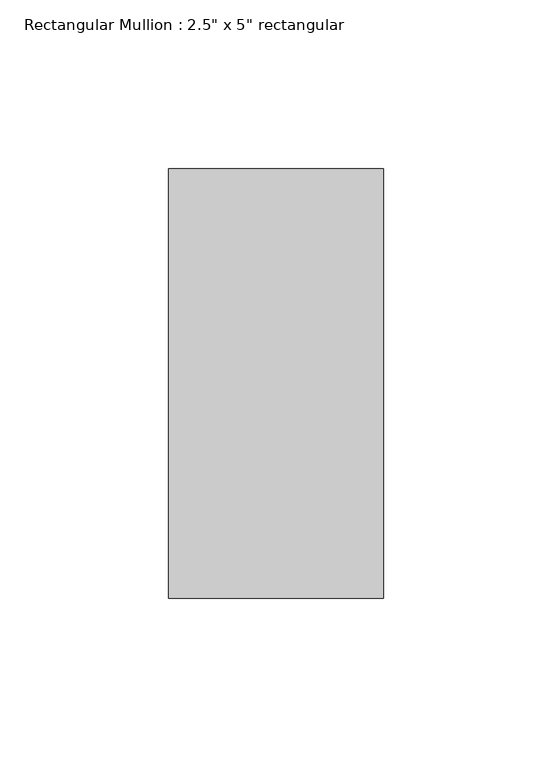
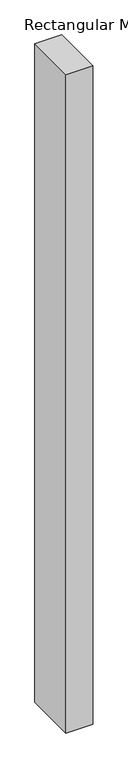
"""IFC4 building model written with IfcOpenShell, lengths in millimetres: member geometry."""

from ifc_helpers import new_model, si_unit, frame, origin, place, context, project, spatial, polyline, outline, extrude, source, transform, mapped, element, save


def member_4a65ca8f(model_context):
    return source(origin(), model_context, "Body", "SweptSolid", [
        extrude(outline(polyline([(0.0, 63.5), (0.0, -63.5), (-63.5, -63.5), (-63.5, 63.5), (0.0, 63.5)])), frame((0.0, 0.0, -1649.5904225), z_axis=(0.0, 0.0, 1.0), x_axis=(1.0, 0.0, 0.0)), (0.0, 0.0, 1.0), 1649.5904225),
    ])


if __name__ == "__main__":
    model = new_model("IFC4")
    model_context = context("Model", 3, world=origin())
    ifc_project = project(units=[si_unit("LENGTHUNIT", "METRE", prefix="MILLI")], contexts=[model_context])
    site = spatial("IfcSite", under=ifc_project)
    building = spatial("IfcBuilding", under=site)
    placement = place(None, origin())
    member_shape = member_4a65ca8f(model_context)
    element("IfcMember", 1, ObjectType="Rectangular Mullion : 2.5\" x 5\" rectangular", at=placement, inside=building, context=model_context, shape_type="MappedRepresentation", body=[
        mapped(member_shape, transform((0.0, 0.0, 0.0), x_axis=(1.0, 0.0, 0.0), y_axis=(0.0, 1.0, 0.0), z_axis=(0.0, 0.0, 1.0))),
    ])
    save(model, "model.ifc")

# Revit data of these elements
# Type "Rectangular Mullion : 2.5\" x 5\" rectangular"
#   built-in parameter 1007304 = 0.416667 (stored number, unit not read)
#   built-in parameter 1007301 = 0.104167 (stored number, unit not read)
#   built-in parameter 1007300 = 0.104167 (stored number, unit not read)
# Element 1 (IfcMember, "Rectangular Mullion : 2.5\" x 5\" rectangular")
#   Materials on its faces: "Aluminum"
# Materials
#   "Aluminum": class "Metal", colour RGB 247 247 247, transparency 0, Description = "Aluminum 6061", Cost = 0
